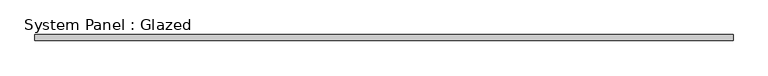
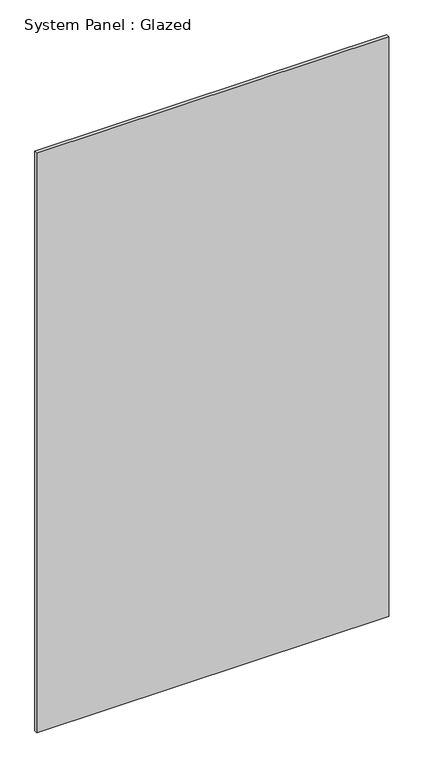
"""IFC4 building model written with IfcOpenShell, lengths in millimetres: plate geometry, System Panel : Glazed."""

from ifc_helpers import new_model, si_unit, origin, origin_with_axes, place, context, project, spatial, polyline, outline, extrude, source, transform, mapped, element, save


def system_panel_glazed_ffaa535b(model_context):
    return source(origin(), model_context, "Body", "SweptSolid", [
        extrude(outline(polyline([(1460.5, 19.05), (-1460.5, 19.05), (-1460.5, 44.45), (1460.5, 44.45), (1460.5, 19.05)])), origin_with_axes(), (0.0, 0.0, 1.0), 5086.35),
    ])


if __name__ == "__main__":
    model = new_model("IFC4")
    model_context = context("Model", 3, world=origin())
    ifc_project = project(units=[si_unit("LENGTHUNIT", "METRE", prefix="MILLI")], contexts=[model_context])
    site = spatial("IfcSite", under=ifc_project)
    building = spatial("IfcBuilding", under=site)
    placement = place(None, origin())
    system_panel_glazed_shape = system_panel_glazed_ffaa535b(model_context)
    element("IfcPlate", 1, ObjectType="System Panel : Glazed", at=placement, inside=building, context=model_context, shape_type="MappedRepresentation", body=[
        mapped(system_panel_glazed_shape, transform((0.0, 0.0, 0.0), x_axis=(1.0, 0.0, 0.0), y_axis=(0.0, 1.0, 0.0), z_axis=(0.0, 0.0, 1.0))),
    ])
    save(model, "model.ifc")

# Revit data of these elements
# Type "System Panel : Glazed"
#   Construction Type Id = "GSP4R"
#   Analytic Construction = "1/8 in Pilkington single glazing"
#   Visual Light Transmittance = 0.9
#   Solar Heat Gain Coefficient = 0.86
#   Heat Transfer Coefficient (U) = 1.18115 BTU/(h·ft²·°F)
# Element 1 (IfcPlate, "System Panel : Glazed")
#   Materials on its faces: "Glass"
# Materials
#   "Glass": class "Glass", colour RGB 0 128 192, transparency 0.75, Description = "Soda Lime Glass", Cost = 0
